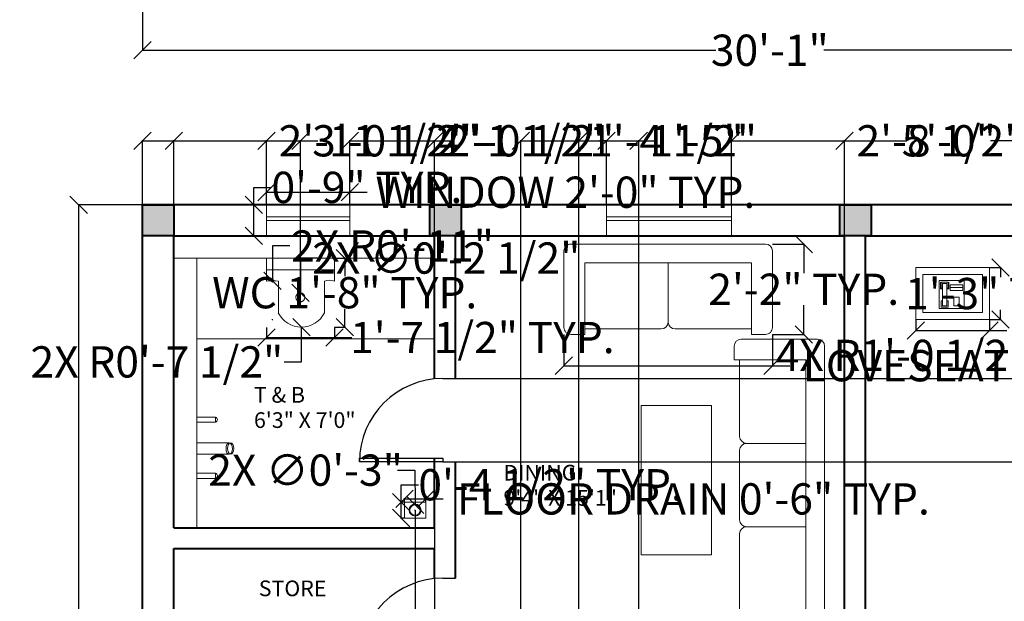
# Model space of a CAD drawing. Units: inches. Extents: x -19 to 1000, y -122 to 1144.
# Tile 2 of 8: x -14 to 270, y 146 to 313. Entities that reach past the tile are written whole.
import ezdxf

# ---------------------------------------------------------------- set-up
doc = ezdxf.new("R2010")
doc.units = ezdxf.units.IN
doc.header["$MEASUREMENT"] = 0
for name, color, linetype, lineweight in [('A-ANNO-DIMS', 191, 'Continuous', 18), ('A-AREA-IDEN', 1, 'Continuous', 18), ('A-COLS', 4, 'Continuous', 40), ('A-COLS-PATT', 220, 'Continuous', 13), ('A-EQPM', 120, 'Continuous', 18), ('A-FLOR-FIXT', 8, 'Continuous', 18), ('DOORS', 2, 'Continuous', 25), ('FURNITURE', 120, 'Continuous', 18), ('WALLS', 4, 'Continuous', 40), ('WINDOWS', 3, 'Continuous', 18)]:
    doc.layers.add(name, color=color, linetype=linetype, lineweight=lineweight)
doc.styles.get("Standard").update_dxf_attribs({"font": 'arial.ttf'})
doc.dimstyles.get("Standard").update_dxf_attribs({"dimtxt": 9, "dimasz": 5, "dimexe": 0.18, "dimexo": 0.0625, "dimgap": 0.09, "dimtad": 0, "dimtih": 1, "dimtoh": 1, "dimdec": 0, "dimzin": 0, "dimdsep": 46, "dimlunit": 3, "dimtxsty": 'Standard', "dimblk": 'OBLIQUE', "dimcen": 0.09, "dimadec": 0, "dimazin": 0, "dimtfac": 1, "dimtdec": 0, "dimtofl": 0, "dimtmove": 0, "dimatfit": 3, "dimfxl": 1, "dimtolj": 1, "dimtzin": 0, "dimarcsym": 0})

# ---------------------------------------------------------------- blocks, each defined once
blk = doc.blocks.new('Phone - Desk')
for p, q in [((-4.5, -5), (-4.5, 5)), ((-4.5, 5), (4.5, 5)), ((-4, 4.5), (-4, 2)), ((-3.75, 4.5), (-3.75, 2.25)), ((-1.25, 4.5), (-3.75, 4.5)), ((-3.25, 4), (-3.25, -4)), ((-3.25, 4), (-1.75, 4)), ((-1.75, -4), (-1.75, 4)), ((-1.25, 2.25), (-1.25, 4.5)), ((-1, 2), (-1, 4.5)), ((4.5, 5), (4.5, -5)), ((-4, 2), (-3.25, 2)), ((-3.75, 2.25), (-3.25, 2.25)), ((-1.75, 2.25), (-1.25, 2.25)), ((-1.75, 2), (-1, 2)), ((4, 3.5), (-0.5, 3.5)), ((-0.5, 3.5), (-0.5, 1.5)), ((-0.5, 2.5), (4, 2.5)), ((-0.5, 1.5), (4, 1.5)), ((4, 1.5), (4, 3.5)), ((-3.75, -2.25), (-3.25, -2.25)), ((-3.75, -4.5), (-3.75, -2.25)), ((-1.75, -2.25), (-1.25, -2.25)), ((-1.25, -2.25), (-1.25, -4.5)), ((2.75, -1), (0.75, -1)), ((0.75, -1), (0.75, -4)), ((2.75, -4), (2.75, -1)), ((4.5, -5), (-4.5, -5)), ((-1.25, -4.5), (-3.75, -4.5)), ((-3.25, -4), (-1.75, -4)), ((0.75, -4), (2.75, -4))]:
    blk.add_line(p, q)
blk = doc.blocks.new('*U3')
for p, q in [((0, 0), (0, -6)), ((40, 0), (40, -6))]:
    blk.add_line(p, q)
blk.add_lwpolyline([(0, 0), (0, 40), (1.75, 40), (1.75, 0)], close=True)
blk.add_arc((0, 0), 40, 0, 90)
blk = doc.blocks.new('SOFA-THREE-SEAT')
for p, q in [((2, 84), (24, 84)), ((0, 78), (0, 82)), ((26, 82), (26, 2)), ((0, 78), (20.62, 78)), ((1.56, 78), (1.56, 56)), ((20.62, 78), (20.62, 6)), ((3.56, 54), (20.62, 54)), ((3.56, 54), (3.56, 54)), ((1.56, 52), (1.56, 32)), ((3.56, 30), (20.62, 30)), ((3.56, 30), (3.56, 30)), ((1.56, 28), (1.56, 6)), ((2, 6), (20.62, 6)), ((0, 2), (0, 4)), ((24, 0), (2, 0))]:
    blk.add_line(p, q)
for centre, start, end in [((2, 82), 90, 180), ((24, 82), 0, 90), ((3.56, 56), 180, 270), ((3.56, 52), 90, 180), ((3.56, 32), 180, 270), ((3.56, 28), 90, 180), ((2, 4), 90, 180), ((2, 2), 180, 270), ((24, 2), 270, 0)]:
    blk.add_arc(centre, 2, start, end)
blk = doc.blocks.new('LOVESEAT')
for p, q in [((6, 20.62), (54, 20.62)), ((6, 0), (6, 20.62)), ((30, 3.56), (30, 20.62)), ((54, 0), (54, 20.62)), ((30, 3.56), (30, 3.56)), ((6, 1.56), (28, 1.56)), ((32, 1.56), (54, 1.56))]:
    blk.add_line(p, q)
blk.add_lwpolyline([(6, 0), (2, 0, -0.414214), (0, 2), (0, 24, -0.414214), (2, 26), (58, 26, -0.414213), (60, 24), (60, 2, -0.414214), (58, 0), (54, 0)], format="xyb")
for centre, start, end in [((28, 3.56), 270, 0), ((32, 3.56), 180, 270)]:
    blk.add_arc(centre, 2, start, end)
blk = doc.blocks.new('TABLE-COFFEE')
blk.add_lwpolyline([(20.25, 0), (0, 0), (0, 43), (20.25, 43)], close=True)
blk = doc.blocks.new('TABLE-BEDSIDE')
for points in [[(0, 0), (21.2, 0), (21.2, 14.94), (0, 14.94)], [(2, 2), (19.2, 2), (19.2, 12.94), (2, 12.94)]]:
    blk.add_lwpolyline(points, close=True)
blk = doc.blocks.new('WC-PLAN')
for p, q in [((0, 13.24), (0, 19.84)), ((0, 19.84), (19.57, 19.84)), ((19.57, 13.24), (19.57, 19.84)), ((0, 16.54), (19.57, 16.54)), ((3.44, 13.24), (3.44, 4.14)), ((16.7, 13.24), (16.7, 4.14))]:
    blk.add_line(p, q)
blk.add_circle((9.78, 8.6), 1.3)
for centre, radius, start, end in [((1.72, 2.24), 11.13, 81.1156, 98.8844), ((18.13, 10.18), 3.38, 64.9191, 115.0809), ((10.07, 7.39), 7.39, 206.0978, 333.9022)]:
    blk.add_arc(centre, radius, start, end)
blk = doc.blocks.new('FLOOR-DRAIN')
blk.add_lwpolyline([(6.19, 0), (0, 0), (0, 4.58), (6.19, 4.58)], close=True)
for radius in [1.73, 1.73, 1.73, 1.49]:
    blk.add_circle((3.09, 2.29), radius)
blk = doc.blocks.new('WIN-24-PLAN')
for p, q in [((0, 4.5), (0, 9)), ((0, 9), (0, 0)), ((24, 9), (24, 0)), ((0, 5.5), (24, 5.5)), ((0, 4.5), (24, 4.5))]:
    blk.add_line(p, q)
blk = doc.blocks.new('WIN-36-PLAN')
for p, q in [((0, 4.5), (0, 9)), ((0, 9), (0, 0)), ((36, 9), (36, 0)), ((0, 5.5), (36, 5.5)), ((0, 5.5), (36, 5.5)), ((0, 4.5), (36, 4.5))]:
    blk.add_line(p, q)
blk = doc.blocks.new('COLUMN-9X9')
blk.add_lwpolyline([(0, 9), (9, 9), (9, 0), (0, 0)], close=True)
blk = doc.blocks.new('_Oblique')
at = {"color": 0, "linetype": 'ByBlock', "lineweight": -2}
blk.add_line((-0.5, -0.5), (0.5, 0.5), dxfattribs=at)
blk = doc.blocks.new('*D43')
at = {"layer": 'A-ANNO-DIMS', "color": 0, "lineweight": -2, "transparency": 16777216}
for p, q in [((244.17, 226.6), (244.17, 223.31)), ((265.37, 226.6), (265.37, 223.31)), ((244.17, 223.49), (265.37, 223.49)), ((265.37, 223.49), (270.37, 223.49))]:
    blk.add_line(p, q, dxfattribs=at)
at = {"layer": 'Defpoints', "color": 0, "transparency": 16777216}
for p in [(244.17, 226.67), (265.37, 226.67), (265.37, 223.49)]:
    blk.add_point(p, dxfattribs=at)
at = {"layer": 'A-ANNO-DIMS', "color": 0, "lineweight": -2, "transparency": 16777216, "xscale": 5, "yscale": 5, "zscale": 5, "rotation": 180}
blk.add_blockref('_Oblique', (244.17, 223.49), dxfattribs=at)
at = {"layer": 'A-ANNO-DIMS', "color": 0, "lineweight": -2, "transparency": 16777216, "xscale": 5, "yscale": 5, "zscale": 5}
blk.add_blockref('_Oblique', (265.37, 223.49), dxfattribs=at)
at = {"layer": 'A-ANNO-DIMS', "color": 0, "transparency": 16777216, "insert": (340.28, 223.49), "char_height": 9, "attachment_point": 5}
blk.add_mtext('\\A1;NIGHTSTAND 1\'-9" TYP.', dxfattribs=at)
blk = doc.blocks.new('*D44')
at = {"layer": 'A-ANNO-DIMS', "color": 0, "lineweight": -2, "transparency": 16777216}
for p, q in [((265.43, 241.6), (268.73, 241.6)), ((268.55, 241.6), (268.55, 238.82)), ((268.55, 226.67), (268.55, 229.45)), ((265.43, 226.67), (268.73, 226.67))]:
    blk.add_line(p, q, dxfattribs=at)
at = {"layer": 'Defpoints', "color": 0, "transparency": 16777216}
for p in [(265.37, 241.6), (268.55, 241.6), (265.37, 226.67)]:
    blk.add_point(p, dxfattribs=at)
at = {"layer": 'A-ANNO-DIMS', "color": 0, "lineweight": -2, "transparency": 16777216, "xscale": 5, "yscale": 5, "zscale": 5}
for p, rotation in [((268.55, 241.6), 90), ((268.55, 226.67), 270)]:
    blk.add_blockref('_Oblique', p, dxfattribs=dict(at, rotation=rotation))
at = {"layer": 'A-ANNO-DIMS', "color": 0, "transparency": 16777216, "insert": (268.55, 234.13), "char_height": 9, "attachment_point": 5}
blk.add_mtext('\\A1;1\'-3" TYP.', dxfattribs=at)
blk = doc.blocks.new('*D55')
at = {"layer": 'A-ANNO-DIMS', "color": 0, "lineweight": -2, "transparency": 16777216}
for p, q in [((142.9, 222.31), (142.9, 213.19)), ((202.9, 222.31), (202.9, 213.19)), ((142.9, 213.37), (202.9, 213.37)), ((202.9, 213.37), (207.9, 213.37))]:
    blk.add_line(p, q, dxfattribs=at)
at = {"layer": 'Defpoints', "color": 0, "transparency": 16777216}
for p in [(142.9, 222.37), (202.9, 222.37), (202.9, 213.37)]:
    blk.add_point(p, dxfattribs=at)
at = {"layer": 'A-ANNO-DIMS', "color": 0, "lineweight": -2, "transparency": 16777216, "xscale": 5, "yscale": 5, "zscale": 5, "rotation": 180}
blk.add_blockref('_Oblique', (142.9, 213.37), dxfattribs=at)
at = {"layer": 'A-ANNO-DIMS', "color": 0, "lineweight": -2, "transparency": 16777216, "xscale": 5, "yscale": 5, "zscale": 5}
blk.add_blockref('_Oblique', (202.9, 213.37), dxfattribs=at)
at = {"layer": 'A-ANNO-DIMS', "color": 0, "transparency": 16777216, "insert": (270.16, 213.37), "char_height": 9, "attachment_point": 5}
blk.add_mtext('\\A1;LOVESEAT 5\'-0" TYP.', dxfattribs=at)
blk = doc.blocks.new('*D56')
at = {"layer": 'A-ANNO-DIMS', "color": 0, "lineweight": -2, "transparency": 16777216}
for p, q in [((202.96, 248.37), (212.08, 248.37)), ((211.9, 248.37), (211.9, 239.99)), ((211.9, 222.37), (211.9, 230.76)), ((202.96, 222.37), (212.08, 222.37))]:
    blk.add_line(p, q, dxfattribs=at)
at = {"layer": 'Defpoints', "color": 0, "transparency": 16777216}
for p in [(202.9, 248.37), (211.9, 248.37), (202.9, 222.37)]:
    blk.add_point(p, dxfattribs=at)
at = {"layer": 'A-ANNO-DIMS', "color": 0, "lineweight": -2, "transparency": 16777216, "xscale": 5, "yscale": 5, "zscale": 5}
for p, rotation in [((211.9, 248.37), 90), ((211.9, 222.37), 270)]:
    blk.add_blockref('_Oblique', p, dxfattribs=dict(at, rotation=rotation))
at = {"layer": 'A-ANNO-DIMS', "color": 0, "transparency": 16777216, "insert": (211.9, 235.37), "char_height": 9, "attachment_point": 5}
blk.add_mtext('\\A1;2\'-2" TYP.', dxfattribs=at)
blk = doc.blocks.new('*D65')
at = {"layer": 'A-ANNO-DIMS', "color": 0, "lineweight": -2, "transparency": 16777216}
for p, q in [((76.9, 244.3), (79.99, 244.3)), ((79.81, 244.3), (79.81, 239.12)), ((79.81, 224.46), (79.81, 229.64)), ((76.9, 224.46), (79.99, 224.46))]:
    blk.add_line(p, q, dxfattribs=at)
at = {"layer": 'Defpoints', "color": 0, "transparency": 16777216}
for p in [(76.84, 244.3), (79.81, 244.3), (76.84, 224.46)]:
    blk.add_point(p, dxfattribs=at)
at = {"layer": 'A-ANNO-DIMS', "color": 0, "lineweight": -2, "transparency": 16777216, "xscale": 5, "yscale": 5, "zscale": 5}
for p, rotation in [((79.81, 244.3), 90), ((79.81, 224.46), 270)]:
    blk.add_blockref('_Oblique', p, dxfattribs=dict(at, rotation=rotation))
at = {"layer": 'A-ANNO-DIMS', "color": 0, "transparency": 16777216, "insert": (79.81, 234.38), "char_height": 9, "attachment_point": 5}
blk.add_mtext('\\A1;WC 1\'-8" TYP.', dxfattribs=at)
blk = doc.blocks.new('*D66')
at = {"layer": 'A-ANNO-DIMS', "color": 0, "lineweight": -2, "transparency": 16777216}
for p, q in [((57.27, 224.4), (57.27, 221.3)), ((76.84, 224.4), (76.84, 221.3)), ((57.27, 221.48), (76.84, 221.48)), ((76.84, 221.48), (81.84, 221.48))]:
    blk.add_line(p, q, dxfattribs=at)
at = {"layer": 'Defpoints', "color": 0, "transparency": 16777216}
for p in [(57.27, 224.46), (76.84, 224.46), (76.84, 221.48)]:
    blk.add_point(p, dxfattribs=at)
at = {"layer": 'A-ANNO-DIMS', "color": 0, "lineweight": -2, "transparency": 16777216, "xscale": 5, "yscale": 5, "zscale": 5, "rotation": 180}
blk.add_blockref('_Oblique', (57.27, 221.48), dxfattribs=at)
at = {"layer": 'A-ANNO-DIMS', "color": 0, "lineweight": -2, "transparency": 16777216, "xscale": 5, "yscale": 5, "zscale": 5}
blk.add_blockref('_Oblique', (76.84, 221.48), dxfattribs=at)
at = {"layer": 'A-ANNO-DIMS', "color": 0, "transparency": 16777216, "insert": (119.42, 221.48), "char_height": 9, "attachment_point": 5}
blk.add_mtext('\\A1;1\'-7 1/2" TYP.', dxfattribs=at)
blk = doc.blocks.new('*D67')
at = {"layer": 'A-ANNO-DIMS', "color": 0, "lineweight": -2, "transparency": 16777216}
for p, q in [((96.97, 174.15), (96.97, 175.2)), ((96.97, 175.02), (103.16, 175.02)), ((103.16, 174.15), (103.16, 175.2)), ((103.16, 175.02), (108.16, 175.02))]:
    blk.add_line(p, q, dxfattribs=at)
at = {"layer": 'Defpoints', "color": 0, "transparency": 16777216}
for p in [(96.97, 174.09), (103.16, 175.02), (103.16, 174.09)]:
    blk.add_point(p, dxfattribs=at)
at = {"layer": 'A-ANNO-DIMS', "color": 0, "lineweight": -2, "transparency": 16777216, "xscale": 5, "yscale": 5, "zscale": 5, "rotation": 180}
blk.add_blockref('_Oblique', (96.97, 175.02), dxfattribs=at)
at = {"layer": 'A-ANNO-DIMS', "color": 0, "lineweight": -2, "transparency": 16777216, "xscale": 5, "yscale": 5, "zscale": 5}
blk.add_blockref('_Oblique', (103.16, 175.02), dxfattribs=at)
at = {"layer": 'A-ANNO-DIMS', "color": 0, "transparency": 16777216, "insert": (180.14, 175.02), "char_height": 9, "attachment_point": 5}
blk.add_mtext('\\A1;FLOOR DRAIN 0\'-6" TYP.', dxfattribs=at)
blk = doc.blocks.new('*D68')
at = {"layer": 'A-ANNO-DIMS', "color": 0, "lineweight": -2, "transparency": 16777216}
for p, q in [((96.05, 174.09), (96.05, 179.09)), ((96.05, 179.09), (101.05, 179.09)), ((96.91, 174.09), (95.87, 174.09)), ((96.05, 169.52), (96.05, 174.09)), ((96.91, 169.52), (95.87, 169.52))]:
    blk.add_line(p, q, dxfattribs=at)
at = {"layer": 'Defpoints', "color": 0, "transparency": 16777216}
for p in [(96.05, 174.09), (96.97, 174.09), (96.97, 169.52)]:
    blk.add_point(p, dxfattribs=at)
at = {"layer": 'A-ANNO-DIMS', "color": 0, "lineweight": -2, "transparency": 16777216, "xscale": 5, "yscale": 5, "zscale": 5}
for p, rotation in [((96.05, 174.09), 90), ((96.05, 169.52), 270)]:
    blk.add_blockref('_Oblique', p, dxfattribs=dict(at, rotation=rotation))
at = {"layer": 'A-ANNO-DIMS', "color": 0, "transparency": 16777216, "insert": (139.05, 179.09), "char_height": 9, "attachment_point": 5}
blk.add_mtext('\\A1;0\'-4 1/2" TYP.', dxfattribs=at)
blk = doc.blocks.new('*D71')
at = {"layer": 'A-ANNO-DIMS', "color": 0, "lineweight": -2, "transparency": 16777216}
for p, q in [((57.27, 259.77), (57.27, 263.49)), ((57.27, 263.31), (81.27, 263.31)), ((81.27, 259.77), (81.27, 263.49)), ((81.27, 263.31), (86.27, 263.31))]:
    blk.add_line(p, q, dxfattribs=at)
at = {"layer": 'Defpoints', "color": 0, "transparency": 16777216}
for p in [(81.27, 263.31), (57.27, 259.71), (81.27, 259.71)]:
    blk.add_point(p, dxfattribs=at)
at = {"layer": 'A-ANNO-DIMS', "color": 0, "lineweight": -2, "transparency": 16777216, "xscale": 5, "yscale": 5, "zscale": 5, "rotation": 180}
blk.add_blockref('_Oblique', (57.27, 263.31), dxfattribs=at)
at = {"layer": 'A-ANNO-DIMS', "color": 0, "lineweight": -2, "transparency": 16777216, "xscale": 5, "yscale": 5, "zscale": 5}
blk.add_blockref('_Oblique', (81.27, 263.31), dxfattribs=at)
at = {"layer": 'A-ANNO-DIMS', "color": 0, "transparency": 16777216, "insert": (143.31, 263.31), "char_height": 9, "attachment_point": 5}
blk.add_mtext('\\A1;WINDOW 2\'-0" TYP.', dxfattribs=at)
blk = doc.blocks.new('*D72')
at = {"layer": 'A-ANNO-DIMS', "color": 0, "lineweight": -2, "transparency": 16777216}
for p, q in [((53.67, 259.71), (53.67, 264.71)), ((53.67, 264.71), (58.67, 264.71)), ((57.21, 259.71), (53.49, 259.71)), ((53.67, 250.71), (53.67, 259.71)), ((57.21, 250.71), (53.49, 250.71))]:
    blk.add_line(p, q, dxfattribs=at)
at = {"layer": 'Defpoints', "color": 0, "transparency": 16777216}
for p in [(53.67, 259.71), (57.27, 259.71), (57.27, 250.71)]:
    blk.add_point(p, dxfattribs=at)
at = {"layer": 'A-ANNO-DIMS', "color": 0, "lineweight": -2, "transparency": 16777216, "xscale": 5, "yscale": 5, "zscale": 5}
for p, rotation in [((53.67, 259.71), 90), ((53.67, 250.71), 270)]:
    blk.add_blockref('_Oblique', p, dxfattribs=dict(at, rotation=rotation))
at = {"layer": 'A-ANNO-DIMS', "color": 0, "transparency": 16777216, "insert": (86.19, 264.71), "char_height": 9, "attachment_point": 5}
blk.add_mtext('\\A1;0\'-9" TYP.', dxfattribs=at)
blk = doc.blocks.new('*D84')
at = {"layer": 'A-ANNO-DIMS', "color": 0, "lineweight": -2, "transparency": 16777216}
for p, q in [((21.58, 259.71), (3.06, 259.71)), ((3.24, 259.71), (3.24, 89.39)), ((3.24, -90.29), (3.24, 80.02)), ((21.58, -90.29), (3.06, -90.29))]:
    blk.add_line(p, q, dxfattribs=at)
at = {"layer": 'Defpoints', "color": 0, "transparency": 16777216}
for p in [(3.24, 259.71), (21.64, 259.71), (21.64, -90.29)]:
    blk.add_point(p, dxfattribs=at)
at = {"layer": 'A-ANNO-DIMS', "color": 0, "lineweight": -2, "transparency": 16777216, "xscale": 5, "yscale": 5, "zscale": 5}
for p, rotation in [((3.24, 259.71), 90), ((3.24, -90.29), 270)]:
    blk.add_blockref('_Oblique', p, dxfattribs=dict(at, rotation=rotation))
at = {"layer": 'A-ANNO-DIMS', "color": 0, "transparency": 16777216, "insert": (3.24, 84.71), "char_height": 9, "attachment_point": 5}
blk.add_mtext('\\A1;29\'-2"', dxfattribs=at)
blk = doc.blocks.new('*D85')
at = {"layer": 'A-ANNO-DIMS', "color": 0, "lineweight": -2, "transparency": 16777216}
for p, q in [((21.64, 259.77), (21.64, 278.29)), ((21.64, 278.11), (57.27, 278.11)), ((57.27, 259.77), (57.27, 278.29)), ((57.27, 278.11), (62.27, 278.11))]:
    blk.add_line(p, q, dxfattribs=at)
at = {"layer": 'Defpoints', "color": 0, "transparency": 16777216}
for p in [(57.27, 278.11), (21.64, 259.71), (57.27, 259.71)]:
    blk.add_point(p, dxfattribs=at)
at = {"layer": 'A-ANNO-DIMS', "color": 0, "lineweight": -2, "transparency": 16777216, "xscale": 5, "yscale": 5, "zscale": 5, "rotation": 180}
blk.add_blockref('_Oblique', (21.64, 278.11), dxfattribs=at)
at = {"layer": 'A-ANNO-DIMS', "color": 0, "lineweight": -2, "transparency": 16777216, "xscale": 5, "yscale": 5, "zscale": 5}
blk.add_blockref('_Oblique', (57.27, 278.11), dxfattribs=at)
at = {"layer": 'A-ANNO-DIMS', "color": 0, "transparency": 16777216, "insert": (88.38, 278.11), "char_height": 9, "attachment_point": 5}
blk.add_mtext('\\A1;2\'-11 1/2"', dxfattribs=at)
blk = doc.blocks.new('*D86')
at = {"layer": 'A-ANNO-DIMS', "color": 0, "lineweight": -2, "transparency": 16777216}
for p, q in [((81.27, 259.77), (81.27, 278.29)), ((81.27, 278.11), (105.64, 278.11)), ((105.64, 250.77), (105.64, 278.29)), ((105.64, 278.11), (110.64, 278.11))]:
    blk.add_line(p, q, dxfattribs=at)
at = {"layer": 'Defpoints', "color": 0, "transparency": 16777216}
for p in [(105.64, 278.11), (81.27, 259.71), (105.64, 250.71)]:
    blk.add_point(p, dxfattribs=at)
at = {"layer": 'A-ANNO-DIMS', "color": 0, "lineweight": -2, "transparency": 16777216, "xscale": 5, "yscale": 5, "zscale": 5, "rotation": 180}
blk.add_blockref('_Oblique', (81.27, 278.11), dxfattribs=at)
at = {"layer": 'A-ANNO-DIMS', "color": 0, "lineweight": -2, "transparency": 16777216, "xscale": 5, "yscale": 5, "zscale": 5}
blk.add_blockref('_Oblique', (105.64, 278.11), dxfattribs=at)
at = {"layer": 'A-ANNO-DIMS', "color": 0, "transparency": 16777216, "insert": (133.26, 278.11), "char_height": 9, "attachment_point": 5}
blk.add_mtext('\\A1;2\'-0 1/2"', dxfattribs=at)
blk = doc.blocks.new('*D87')
at = {"layer": 'A-ANNO-DIMS', "color": 0, "lineweight": -2, "transparency": 16777216}
for p, q in [((105.64, 250.77), (105.64, 278.29)), ((105.64, 278.11), (107.68, 278.11)), ((155.15, 278.11), (153.12, 278.11)), ((155.15, 259.77), (155.15, 278.29))]:
    blk.add_line(p, q, dxfattribs=at)
at = {"layer": 'Defpoints', "color": 0, "transparency": 16777216}
for p in [(155.15, 278.11), (155.15, 259.71), (105.64, 250.71)]:
    blk.add_point(p, dxfattribs=at)
at = {"layer": 'A-ANNO-DIMS', "color": 0, "lineweight": -2, "transparency": 16777216, "xscale": 5, "yscale": 5, "zscale": 5, "rotation": 180}
blk.add_blockref('_Oblique', (105.64, 278.11), dxfattribs=at)
at = {"layer": 'A-ANNO-DIMS', "color": 0, "lineweight": -2, "transparency": 16777216, "xscale": 5, "yscale": 5, "zscale": 5}
blk.add_blockref('_Oblique', (155.15, 278.11), dxfattribs=at)
at = {"layer": 'A-ANNO-DIMS', "color": 0, "transparency": 16777216, "insert": (130.4, 278.11), "char_height": 9, "attachment_point": 5}
blk.add_mtext('\\A1;4\'-1 1/2"', dxfattribs=at)
blk = doc.blocks.new('*D88')
at = {"layer": 'A-ANNO-DIMS', "color": 0, "lineweight": -2, "transparency": 16777216}
for p, q in [((191.15, 259.77), (191.15, 278.29)), ((191.15, 278.11), (223.64, 278.11)), ((223.64, 250.77), (223.64, 278.29)), ((223.64, 278.11), (228.64, 278.11))]:
    blk.add_line(p, q, dxfattribs=at)
at = {"layer": 'Defpoints', "color": 0, "transparency": 16777216}
for p in [(223.64, 278.11), (191.15, 259.71), (223.64, 250.71)]:
    blk.add_point(p, dxfattribs=at)
at = {"layer": 'A-ANNO-DIMS', "color": 0, "lineweight": -2, "transparency": 16777216, "xscale": 5, "yscale": 5, "zscale": 5, "rotation": 180}
blk.add_blockref('_Oblique', (191.15, 278.11), dxfattribs=at)
at = {"layer": 'A-ANNO-DIMS', "color": 0, "lineweight": -2, "transparency": 16777216, "xscale": 5, "yscale": 5, "zscale": 5}
blk.add_blockref('_Oblique', (223.64, 278.11), dxfattribs=at)
at = {"layer": 'A-ANNO-DIMS', "color": 0, "transparency": 16777216, "insert": (251.26, 278.11), "char_height": 9, "attachment_point": 5}
blk.add_mtext('\\A1;2\'-8 1/2"', dxfattribs=at)
blk = doc.blocks.new('*D89')
at = {"layer": 'A-ANNO-DIMS', "color": 0, "lineweight": -2, "transparency": 16777216}
for p, q in [((223.64, 250.77), (223.64, 278.29)), ((223.64, 278.11), (241.59, 278.11)), ((283.63, 278.11), (265.69, 278.11)), ((283.63, 259.77), (283.63, 278.29))]:
    blk.add_line(p, q, dxfattribs=at)
at = {"layer": 'Defpoints', "color": 0, "transparency": 16777216}
for p in [(283.63, 278.11), (283.63, 259.71), (223.64, 250.71)]:
    blk.add_point(p, dxfattribs=at)
at = {"layer": 'A-ANNO-DIMS', "color": 0, "lineweight": -2, "transparency": 16777216, "xscale": 5, "yscale": 5, "zscale": 5, "rotation": 180}
blk.add_blockref('_Oblique', (223.64, 278.11), dxfattribs=at)
at = {"layer": 'A-ANNO-DIMS', "color": 0, "lineweight": -2, "transparency": 16777216, "xscale": 5, "yscale": 5, "zscale": 5}
blk.add_blockref('_Oblique', (283.63, 278.11), dxfattribs=at)
at = {"layer": 'A-ANNO-DIMS', "color": 0, "transparency": 16777216, "insert": (253.64, 278.11), "char_height": 9, "attachment_point": 5}
blk.add_mtext('\\A1;5\'-0"', dxfattribs=at)
blk = doc.blocks.new('*D97')
at = {"layer": 'A-ANNO-DIMS', "color": 0, "lineweight": -2, "transparency": 16777216}
for p, q in [((111.7, 209.69), (401.22, 209.69)), ((401.04, 209.69), (401.04, 202.37)), ((401.04, 185.69), (401.04, 193)), ((111.7, 185.69), (401.22, 185.69))]:
    blk.add_line(p, q, dxfattribs=at)
at = {"layer": 'Defpoints', "color": 0, "transparency": 16777216}
for p in [(111.64, 209.69), (401.04, 209.69), (111.64, 185.69)]:
    blk.add_point(p, dxfattribs=at)
at = {"layer": 'A-ANNO-DIMS', "color": 0, "lineweight": -2, "transparency": 16777216, "xscale": 5, "yscale": 5, "zscale": 5}
for p, rotation in [((401.04, 209.69), 90), ((401.04, 185.69), 270)]:
    blk.add_blockref('_Oblique', p, dxfattribs=dict(at, rotation=rotation))
at = {"layer": 'A-ANNO-DIMS', "color": 0, "transparency": 16777216, "insert": (401.04, 197.69), "char_height": 9, "attachment_point": 5}
blk.add_mtext('\\A1;2\'-0"', dxfattribs=at)
blk = doc.blocks.new('*D98')
at = {"layer": 'A-ANNO-DIMS', "color": 0, "lineweight": -2, "transparency": 16777216}
for p, q in [((30.64, 250.77), (30.64, 278.29)), ((30.64, 278.11), (67.06, 278.11)), ((67.06, 233.12), (67.06, 278.29)), ((67.06, 278.11), (72.06, 278.11))]:
    blk.add_line(p, q, dxfattribs=at)
at = {"layer": 'Defpoints', "color": 0, "transparency": 16777216}
for p in [(67.06, 278.11), (30.64, 250.71), (67.06, 233.05)]:
    blk.add_point(p, dxfattribs=at)
at = {"layer": 'A-ANNO-DIMS', "color": 0, "lineweight": -2, "transparency": 16777216, "xscale": 5, "yscale": 5, "zscale": 5, "rotation": 180}
blk.add_blockref('_Oblique', (30.64, 278.11), dxfattribs=at)
at = {"layer": 'A-ANNO-DIMS', "color": 0, "lineweight": -2, "transparency": 16777216, "xscale": 5, "yscale": 5, "zscale": 5}
blk.add_blockref('_Oblique', (67.06, 278.11), dxfattribs=at)
at = {"layer": 'A-ANNO-DIMS', "color": 0, "transparency": 16777216, "insert": (94.59, 278.11), "char_height": 9, "attachment_point": 5}
blk.add_mtext('\\A1;3\'-0 1/2"', dxfattribs=at)
blk = doc.blocks.new('*D99')
at = {"layer": 'A-ANNO-DIMS', "color": 0, "lineweight": -2, "transparency": 16777216}
for p, q in [((105.7, 250.71), (401.22, 250.71)), ((401.04, 250.71), (401.04, 234.89)), ((401.04, 209.69), (401.04, 225.51)), ((111.7, 209.69), (401.22, 209.69))]:
    blk.add_line(p, q, dxfattribs=at)
at = {"layer": 'Defpoints', "color": 0, "transparency": 16777216}
for p in [(105.64, 250.71), (401.04, 250.71), (111.64, 209.69)]:
    blk.add_point(p, dxfattribs=at)
at = {"layer": 'A-ANNO-DIMS', "color": 0, "lineweight": -2, "transparency": 16777216, "xscale": 5, "yscale": 5, "zscale": 5}
for p, rotation in [((401.04, 250.71), 90), ((401.04, 209.69), 270)]:
    blk.add_blockref('_Oblique', p, dxfattribs=dict(at, rotation=rotation))
at = {"layer": 'A-ANNO-DIMS', "color": 0, "transparency": 16777216, "insert": (401.04, 230.2), "char_height": 9, "attachment_point": 5}
blk.add_mtext('\\A1;3\'-5"', dxfattribs=at)
blk = doc.blocks.new('*D100')
at = {"layer": 'A-ANNO-DIMS', "color": 0, "lineweight": -2, "transparency": 16777216}
for p, q in [((100.07, 171.74), (100.07, -108.87)), ((105.64, 166.64), (105.64, -108.87)), ((100.07, -108.69), (105.64, -108.69)), ((105.64, -108.69), (110.64, -108.69))]:
    blk.add_line(p, q, dxfattribs=at)
at = {"layer": 'Defpoints', "color": 0, "transparency": 16777216}
for p in [(100.07, 171.8), (105.64, 166.71), (105.64, -108.69)]:
    blk.add_point(p, dxfattribs=at)
at = {"layer": 'A-ANNO-DIMS', "color": 0, "lineweight": -2, "transparency": 16777216, "xscale": 5, "yscale": 5, "zscale": 5, "rotation": 180}
blk.add_blockref('_Oblique', (100.07, -108.69), dxfattribs=at)
at = {"layer": 'A-ANNO-DIMS', "color": 0, "lineweight": -2, "transparency": 16777216, "xscale": 5, "yscale": 5, "zscale": 5}
blk.add_blockref('_Oblique', (105.64, -108.69), dxfattribs=at)
at = {"layer": 'A-ANNO-DIMS', "color": 0, "transparency": 16777216, "insert": (133.18, -108.69), "char_height": 9, "attachment_point": 5}
blk.add_mtext('\\A1;0\'-5 1/2"', dxfattribs=at)
blk = doc.blocks.new('*D101')
at = {"layer": 'A-ANNO-DIMS', "color": 0, "lineweight": -2, "transparency": 16777216}
for p, q in [((130.52, 116.04), (130.52, 278.29)), ((130.52, 278.11), (147.19, 278.11)), ((147.19, 116.04), (147.19, 278.29)), ((147.19, 278.11), (152.19, 278.11))]:
    blk.add_line(p, q, dxfattribs=at)
at = {"layer": 'Defpoints', "color": 0, "transparency": 16777216}
for p in [(147.19, 278.11), (130.52, 115.98), (147.19, 115.98)]:
    blk.add_point(p, dxfattribs=at)
at = {"layer": 'A-ANNO-DIMS', "color": 0, "lineweight": -2, "transparency": 16777216, "xscale": 5, "yscale": 5, "zscale": 5, "rotation": 180}
blk.add_blockref('_Oblique', (130.52, 278.11), dxfattribs=at)
at = {"layer": 'A-ANNO-DIMS', "color": 0, "lineweight": -2, "transparency": 16777216, "xscale": 5, "yscale": 5, "zscale": 5}
blk.add_blockref('_Oblique', (147.19, 278.11), dxfattribs=at)
at = {"layer": 'A-ANNO-DIMS', "color": 0, "transparency": 16777216, "insert": (174.3, 278.11), "char_height": 9, "attachment_point": 5}
blk.add_mtext('\\A1;1\'-4 1/2"', dxfattribs=at)
blk = doc.blocks.new('*D102')
at = {"layer": 'A-ANNO-DIMS', "color": 0, "lineweight": -2, "transparency": 16777216}
for p, q in [((147.19, 116.04), (147.19, 278.29)), ((147.19, 278.11), (164.4, 278.11)), ((164.4, 116.04), (164.4, 278.29)), ((164.4, 278.11), (169.4, 278.11))]:
    blk.add_line(p, q, dxfattribs=at)
at = {"layer": 'Defpoints', "color": 0, "transparency": 16777216}
for p in [(164.4, 278.11), (147.19, 115.98), (164.4, 115.98)]:
    blk.add_point(p, dxfattribs=at)
at = {"layer": 'A-ANNO-DIMS', "color": 0, "lineweight": -2, "transparency": 16777216, "xscale": 5, "yscale": 5, "zscale": 5, "rotation": 180}
blk.add_blockref('_Oblique', (147.19, 278.11), dxfattribs=at)
at = {"layer": 'A-ANNO-DIMS', "color": 0, "lineweight": -2, "transparency": 16777216, "xscale": 5, "yscale": 5, "zscale": 5}
blk.add_blockref('_Oblique', (164.4, 278.11), dxfattribs=at)
at = {"layer": 'A-ANNO-DIMS', "color": 0, "transparency": 16777216, "insert": (181.03, 278.11), "char_height": 9, "attachment_point": 5}
blk.add_mtext('\\A1;1\'-5"', dxfattribs=at)
blk = doc.blocks.new('*D111')
at = {"layer": 'A-ANNO-DIMS', "color": 0, "lineweight": -2, "transparency": 16777216}
for p, q in [((21.64, 328.07), (21.64, 304)), ((382.64, 328.07), (382.64, 304)), ((21.64, 304.18), (186.6, 304.18)), ((382.64, 304.18), (217.69, 304.18))]:
    blk.add_line(p, q, dxfattribs=at)
at = {"layer": 'Defpoints', "color": 0, "transparency": 16777216}
for p in [(21.64, 328.13), (382.64, 328.13), (21.64, 304.18)]:
    blk.add_point(p, dxfattribs=at)
at = {"layer": 'A-ANNO-DIMS', "color": 0, "lineweight": -2, "transparency": 16777216, "xscale": 5, "yscale": 5, "zscale": 5, "rotation": 180}
blk.add_blockref('_Oblique', (21.64, 304.18), dxfattribs=at)
at = {"layer": 'A-ANNO-DIMS', "color": 0, "lineweight": -2, "transparency": 16777216, "xscale": 5, "yscale": 5, "zscale": 5}
blk.add_blockref('_Oblique', (382.64, 304.18), dxfattribs=at)
at = {"layer": 'A-ANNO-DIMS', "color": 0, "transparency": 16777216, "insert": (202.14, 304.18), "char_height": 9, "attachment_point": 5}
blk.add_mtext('\\A1;30\'-1"', dxfattribs=at)
blk = doc.blocks.new('*D141')
at = {"layer": 'A-ANNO-DIMS', "color": 0, "lineweight": -2, "transparency": 16777216}
for p, q in [((67.09, 244.35), (67.06, 234.35)), ((72.09, 244.35), (67.09, 244.35)), ((66.97, 233.05), (67.15, 233.05)), ((67.06, 232.96), (67.06, 233.14))]:
    blk.add_line(p, q, dxfattribs=at)
at = {"layer": 'Defpoints', "color": 0, "transparency": 16777216}
for p in [(67.06, 234.35), (67.05, 231.76)]:
    blk.add_point(p, dxfattribs=at)
at = {"layer": 'A-ANNO-DIMS', "color": 0, "lineweight": -2, "transparency": 16777216, "xscale": 5, "yscale": 5, "zscale": 5, "rotation": 269.8002160768907}
blk.add_blockref('_Oblique', (67.06, 234.35), dxfattribs=at)
at = {"layer": 'A-ANNO-DIMS', "color": 0, "transparency": 16777216, "insert": (109.04, 244.35), "char_height": 9, "attachment_point": 5}
blk.add_mtext('\\A1;2X ∅0\'-2 1/2"', dxfattribs=at)
blk = doc.blocks.new('*D142')
at = {"layer": 'A-ANNO-DIMS', "color": 0, "lineweight": -2, "transparency": 16777216}
for p, q in [((94.99, 183.29), (99.99, 183.29)), ((99.99, 183.29), (100.06, 173.29)), ((99.98, 171.8), (100.16, 171.8)), ((100.07, 171.71), (100.07, 171.89))]:
    blk.add_line(p, q, dxfattribs=at)
at = {"layer": 'Defpoints', "color": 0, "transparency": 16777216}
for p in [(100.06, 173.29), (100.08, 170.31)]:
    blk.add_point(p, dxfattribs=at)
at = {"layer": 'A-ANNO-DIMS', "color": 0, "lineweight": -2, "transparency": 16777216, "xscale": 5, "yscale": 5, "zscale": 5, "rotation": 270.3908476855887}
blk.add_blockref('_Oblique', (100.06, 173.29), dxfattribs=at)
at = {"layer": 'A-ANNO-DIMS', "color": 0, "transparency": 16777216, "insert": (68.54, 183.29), "char_height": 9, "attachment_point": 5}
blk.add_mtext('\\A1;2X ∅0\'-3"', dxfattribs=at)
blk = doc.blocks.new('*D143')
at = {"layer": 'A-ANNO-DIMS', "color": 0, "lineweight": -2, "transparency": 16777216}
for p, q in [((67.25, 231.84), (67.43, 231.84)), ((67.34, 231.75), (67.34, 231.93)), ((67.34, 214.46), (67.34, 224.46)), ((62.34, 214.46), (67.34, 214.46))]:
    blk.add_line(p, q, dxfattribs=at)
at = {"layer": 'Defpoints', "color": 0, "transparency": 16777216}
for p in [(67.34, 231.84), (67.34, 224.46)]:
    blk.add_point(p, dxfattribs=at)
at = {"layer": 'A-ANNO-DIMS', "color": 0, "lineweight": -2, "transparency": 16777216, "xscale": 5, "yscale": 5, "zscale": 5, "rotation": 89.99762602879655}
blk.add_blockref('_Oblique', (67.34, 224.46), dxfattribs=at)
at = {"layer": 'A-ANNO-DIMS', "color": 0, "transparency": 16777216, "insert": (25.75, 214.46), "char_height": 9, "attachment_point": 5}
blk.add_mtext('\\A1;2X R0\'-7 1/2"', dxfattribs=at)
blk = doc.blocks.new('*D144')
at = {"layer": 'A-ANNO-DIMS', "color": 0, "lineweight": -2, "transparency": 16777216}
for p, q in [((63.99, 247.83), (58.99, 247.83)), ((58.99, 247.83), (58.99, 237.83)), ((58.9, 226.7), (59.08, 226.7)), ((58.99, 226.61), (58.99, 226.79))]:
    blk.add_line(p, q, dxfattribs=at)
at = {"layer": 'Defpoints', "color": 0, "transparency": 16777216}
for p in [(58.99, 237.83), (58.99, 226.7)]:
    blk.add_point(p, dxfattribs=at)
at = {"layer": 'A-ANNO-DIMS', "color": 0, "lineweight": -2, "transparency": 16777216, "xscale": 5, "yscale": 5, "zscale": 5, "rotation": 269.9988573418093}
blk.add_blockref('_Oblique', (58.99, 237.83), dxfattribs=at)
at = {"layer": 'A-ANNO-DIMS', "color": 0, "transparency": 16777216, "insert": (93.59, 247.83), "char_height": 9, "attachment_point": 5}
blk.add_mtext('\\A1;2X R0\'-11"', dxfattribs=at)
blk = doc.blocks.new('*D148')
at = {"layer": 'A-ANNO-DIMS', "color": 0, "lineweight": -2, "transparency": 16777216}
for p, q in [((276.9, 216.33), (281.9, 216.33)), ((281.9, 216.33), (281.9, 206.33)), ((281.81, 193.63), (281.99, 193.63)), ((281.9, 193.54), (281.9, 193.72))]:
    blk.add_line(p, q, dxfattribs=at)
at = {"layer": 'Defpoints', "color": 0, "transparency": 16777216}
for p in [(281.9, 206.33), (281.9, 193.63)]:
    blk.add_point(p, dxfattribs=at)
at = {"layer": 'A-ANNO-DIMS', "color": 0, "lineweight": -2, "transparency": 16777216, "xscale": 5, "yscale": 5, "zscale": 5, "rotation": 270.0006769551681}
blk.add_blockref('_Oblique', (281.9, 206.33), dxfattribs=at)
at = {"layer": 'A-ANNO-DIMS', "color": 0, "transparency": 16777216, "insert": (240.2, 216.33), "char_height": 9, "attachment_point": 5}
blk.add_mtext('\\A1;4X R1\'-0 1/2"', dxfattribs=at)

msp = doc.modelspace()

# ---------------------------------------------------------------- hatches: boundary and pattern name
at = {"layer": 'A-COLS-PATT'}
h = msp.add_hatch(color=256, dxfattribs=at)
h.dxf.hatch_style = 1
h.paths.add_polyline_path([(30.64, 259.71), (21.64, 259.71), (21.64, 250.71), (30.64, 250.71)])
h.paths.add_polyline_path([(113.34, 259.71), (104.34, 259.71), (104.34, 250.71), (113.34, 250.71)])
h.paths.add_polyline_path([(231.33, 259.71), (222.33, 259.71), (222.33, 250.71), (223.64, 250.71), (231.33, 250.71)])
h.paths.add_polyline_path([(382.64, 259.71), (373.64, 259.71), (373.64, 250.71), (382.64, 250.71)])
h.paths.add_polyline_path([(382.64, 124.35), (373.64, 124.35), (373.64, 115.35), (382.64, 115.35)])
h.paths.add_polyline_path([(382.64, -48.29), (373.64, -48.29), (373.64, -57.29), (382.64, -57.29)])
h.paths.add_polyline_path([(111.64, -48.29), (105.64, -48.29), (105.64, -57.29), (111.64, -57.29)])
h.paths.add_polyline_path([(30.64, -48.11), (21.64, -48.11), (21.64, -57.11), (30.64, -57.11)])
h.paths.add_polyline_path([(30.64, 124.5), (21.64, 124.5), (21.64, 115.5), (30.64, 115.5)])
h.paths.add_polyline_path([(111.64, 122.71), (105.64, 122.71), (105.64, 116.71), (111.64, 116.71)])
h.paths.add_polyline_path([(229.64, 122.71), (223.64, 122.71), (223.64, 116.71), (229.64, 116.71)])
h.paths.add_polyline_path([(229.64, -48.29), (223.64, -48.29), (223.64, -57.29), (229.64, -57.29)])

# ---------------------------------------------------------------- linework, layer by layer
at = {"layer": 'A-FLOR-FIXT'}
for p, q in [((30.64, 244.3), (105.64, 244.3)), ((37.26, 166.71), (37.26, 244.3)), ((37.26, 221.07), (105.64, 221.07)), ((37.26, 198.59), (42.62, 198.59)), ((42.62, 198.59), (42.62, 197.08)), ((37.26, 197.08), (42.62, 197.08)), ((37.26, 191.12), (46.57, 191.12)), ((37.26, 187.85), (46.57, 187.85)), ((37.26, 182.45), (42.62, 182.45)), ((42.62, 182.45), (42.62, 180.94)), ((37.26, 180.94), (42.62, 180.94))]:
    msp.add_line(p, q, dxfattribs=at)
for centre in [(42.4, 197.83), (42.4, 181.69)]:
    msp.add_arc(centre, 0.786, 286.4895, 73.5105, dxfattribs=at)
for centre in [(46.57, 189.48), (46.97, 189.54)]:
    msp.add_ellipse(centre, major_axis=(0, 1.63), ratio=0.555125, dxfattribs=at)
at = {"layer": 'WALLS'}
for p, q in [((21.64, -90.29), (21.64, 259.71)), ((382.64, 259.71), (21.64, 259.71)), ((30.64, 250.71), (105.64, 250.71)), ((30.64, 166.71), (30.64, 250.71)), ((105.64, 209.57), (105.64, 250.71)), ((111.64, 250.71), (223.64, 250.71)), ((111.64, 209.69), (111.64, 250.71)), ((223.64, 112.97), (223.64, 250.71)), ((229.64, 250.71), (373.64, 250.71)), ((229.64, 122.71), (229.64, 250.71)), ((105.64, 166.71), (105.64, 186.74)), ((111.64, 152.21), (111.64, 185.69)), ((30.64, 166.71), (105.64, 166.71)), ((30.64, 160.71), (105.64, 160.71)), ((30.64, 122.71), (30.64, 160.71)), ((105.64, 152.09), (105.64, 160.71))]:
    msp.add_line(p, q, dxfattribs=at)
msp.add_lwpolyline([(111.64, 160.71), (111.64, 160.71), (111.64, 166.71)], dxfattribs=at)

# ---------------------------------------------------------------- block references
at = {"layer": 'A-COLS'}
for p in [(21.64, 250.71), (104.34, 250.71), (222.33, 250.71)]:
    msp.add_blockref('COLUMN-9X9', p, dxfattribs=at)
at = {"layer": 'A-EQPM', "xscale": 0.8015722193121366, "yscale": 0.8015722193121366, "zscale": 0.8015722193121366}
msp.add_blockref('Phone - Desk', (254.47, 233.85), dxfattribs=at)
at = {"layer": 'A-FLOR-FIXT'}
for name, p in [('WC-PLAN', (57.27, 224.46)), ('FLOOR-DRAIN', (96.97, 169.51))]:
    msp.add_blockref(name, p, dxfattribs=at)
at = {"layer": 'DOORS', "xscale": 0.6, "yscale": 0.6, "zscale": 0.6, "rotation": 90}
for p in [(108.04, 185.69), (108.04, 128.21)]:
    msp.add_blockref('*U3', p, dxfattribs=at)
at = {"layer": 'FURNITURE'}
for name, p in [('LOVESEAT', (142.9, 222.38)), ('TABLE-BEDSIDE', (244.17, 226.67)), ('SOFA-THREE-SEAT', (191.9, 137.01)), ('TABLE-COFFEE', (165.09, 158.87))]:
    msp.add_blockref(name, p, dxfattribs=at)
at = {"layer": 'WINDOWS'}
for name, p in [('WIN-24-PLAN', (57.27, 250.71)), ('WIN-36-PLAN', (155.15, 250.71))]:
    msp.add_blockref(name, p, dxfattribs=at)

# ---------------------------------------------------------------- texts
at = {"layer": 'A-AREA-IDEN'}
for s, height, p in [('T & B', 4.516, (53.69, 202.71)), ('6\'3" X 7\'0"', 4.5155, (53.69, 195.45)), ('DINING', 4.516, (125.49, 180.31)), ('9\'4" X 15\'1"', 4.5155, (125.49, 173.05)), (' STORE', 4.516, (53.69, 147.01))]:
    msp.add_text(s, height=height, dxfattribs=at).set_placement(p)

# ---------------------------------------------------------------- dimensions: what is measured, and where the dimension line sits
at = {"layer": 'A-ANNO-DIMS'}
for base, p1, p2, angle, picture, middle in [((21.64, 304.18), (382.64, 328.13), (21.64, 328.13), 180, '*D111', (202.14, 304.18)), ((3.24, 259.71), (21.64, -90.29), (21.64, 259.71), 90, '*D84', (3.24, 84.71)), ((401.04, 250.71), (111.64, 209.69), (105.64, 250.71), 90, '*D99', (401.04, 230.2)), ((401.04, 209.69), (111.64, 185.69), (111.64, 209.69), 90, '*D97', (401.04, 197.69))]:
    dim = msp.add_linear_dim(base=base, p1=p1, p2=p2, angle=angle, dimstyle='Standard', override={"dimdec": 1, "dimlfac": 1, "dimrnd": 0, "dimzin": 1, "dimdsep": 46, "dimlunit": 4, "dimfrac": 2}, dxfattribs=at)
    dim.commit()
    dim.dimension.update_dxf_attribs({"geometry": picture, "text_midpoint": middle})
for base, p1, p2, picture, middle in [((57.27, 278.11), (21.64, 259.71), (57.27, 259.71), '*D85', (88.38, 278.11)), ((67.06, 278.11), (30.64, 250.71), (67.06, 233.05), '*D98', (94.59, 278.11)), ((105.64, 278.11), (81.27, 259.71), (105.64, 250.71), '*D86', (133.26, 278.11)), ((155.15, 278.11), (105.64, 250.71), (155.15, 259.71), '*D87', (130.4, 278.11)), ((147.19, 278.11), (130.52, 115.98), (147.19, 115.98), '*D101', (174.3, 278.11)), ((223.64, 278.11), (191.15, 259.71), (223.64, 250.71), '*D88', (251.26, 278.11)), ((164.4, 278.11), (147.19, 115.98), (164.4, 115.98), '*D102', (181.03, 278.11)), ((283.63, 278.11), (223.64, 250.71), (283.63, 259.71), '*D89', (253.64, 278.11)), ((105.64, -108.69), (100.07, 171.8), (105.64, 166.71), '*D100', (133.18, -108.69))]:
    dim = msp.add_linear_dim(base=base, p1=p1, p2=p2, dimstyle='Standard', override={"dimdec": 1, "dimlfac": 1, "dimrnd": 0, "dimzin": 1, "dimdsep": 46, "dimlunit": 4, "dimfrac": 2}, dxfattribs=at)
    dim.commit()
    dim.dimension.update_dxf_attribs({"geometry": picture, "text_midpoint": middle})
for base, p1, p2, text, picture, middle in [((81.27, 263.31), (57.27, 259.71), (81.27, 259.71), 'WINDOW <> TYP.', '*D71', (143.31, 263.31)), ((265.37, 223.49), (244.17, 226.67), (265.37, 226.67), 'NIGHTSTAND <> TYP.', '*D43', (340.28, 223.49)), ((76.84, 221.48), (57.27, 224.46), (76.84, 224.46), '<> TYP.', '*D66', (119.42, 221.48)), ((202.9, 213.37), (142.9, 222.37), (202.9, 222.37), 'LOVESEAT <> TYP.', '*D55', (270.16, 213.37)), ((103.16, 175.02), (96.97, 174.09), (103.16, 174.09), 'FLOOR DRAIN <> TYP.', '*D67', (180.14, 175.02))]:
    dim = msp.add_linear_dim(base=base, p1=p1, p2=p2, text=text, dimstyle='Standard', override={"dimdec": 1, "dimlfac": 1, "dimrnd": 0, "dimzin": 1, "dimdsep": 46, "dimlunit": 4, "dimfrac": 2}, dxfattribs=at)
    dim.commit()
    dim.dimension.update_dxf_attribs({"geometry": picture, "text_midpoint": middle})
for base, p1, p2, text, picture, middle in [((53.67, 259.71), (57.27, 250.71), (57.27, 259.71), '<> TYP.', '*D72', (86.19, 264.71)), ((79.81, 244.3), (76.84, 224.46), (76.84, 244.3), 'WC <> TYP.', '*D65', (79.81, 234.38)), ((211.9, 248.37), (202.9, 222.37), (202.9, 248.37), '<> TYP.', '*D56', (211.9, 235.37)), ((268.55, 241.6), (265.37, 226.67), (265.37, 241.6), '<> TYP.', '*D44', (268.55, 234.13)), ((96.05, 174.09), (96.97, 169.52), (96.97, 174.09), '<> TYP.', '*D68', (139.05, 179.09))]:
    dim = msp.add_linear_dim(base=base, p1=p1, p2=p2, angle=90, text=text, dimstyle='Standard', override={"dimdec": 1, "dimlfac": 1, "dimrnd": 0, "dimzin": 1, "dimdsep": 46, "dimlunit": 4, "dimfrac": 2}, dxfattribs=at)
    dim.commit()
    dim.dimension.update_dxf_attribs({"geometry": picture, "text_midpoint": middle})
for p1, p2, picture, middle in [((67.05, 231.76), (67.06, 234.35), '*D141', (109.04, 244.35)), ((100.08, 170.31), (100.06, 173.29), '*D142', (68.54, 183.29))]:
    dim = msp.add_diameter_dim_2p(p1=p1, p2=p2, text='2X <>', dimstyle='Standard', override={"dimdec": 1, "dimlfac": 1, "dimrnd": 0, "dimzin": 1, "dimdsep": 46, "dimlunit": 4, "dimfrac": 2}, dxfattribs=at)
    dim.commit()
    dim.dimension.update_dxf_attribs({"geometry": picture, "text_midpoint": middle, "dimtype": 163})
for center, mpoint, text, picture, middle in [((58.99, 226.7), (58.99, 237.83), '2X <>', '*D144', (93.59, 247.83)), ((67.34, 231.84), (67.34, 224.46), '2X <>', '*D143', (25.75, 214.46)), ((281.9, 193.63), (281.9, 206.33), '4X <>', '*D148', (240.2, 216.33))]:
    dim = msp.add_radius_dim(center=center, mpoint=mpoint, text=text, dimstyle='Standard', override={"dimdec": 1, "dimlfac": 1, "dimrnd": 0, "dimzin": 1, "dimdsep": 46, "dimlunit": 4, "dimfrac": 2}, dxfattribs=at)
    dim.commit()
    dim.dimension.update_dxf_attribs({"geometry": picture, "text_midpoint": middle})

doc.saveas('drawing.dxf')
